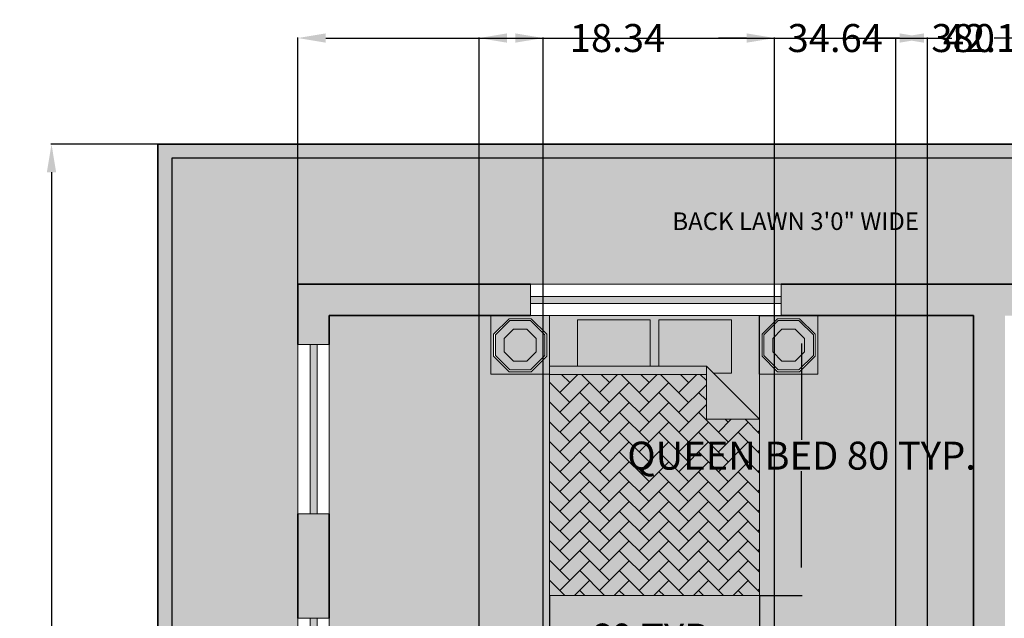
# Model space of a CAD drawing. Units: inches. Extents: x 389 to 971, y 148 to 870.
# Tile 11 of 14: x 389 to 670, y 699 to 870. Entities that reach past the tile are written whole.
import ezdxf

# ---------------------------------------------------------------- set-up
doc = ezdxf.new("R2010")
doc.units = ezdxf.units.IN
doc.header["$MEASUREMENT"] = 0
for name, color, linetype, lineweight in [('A-ANNO-DIMS', 2, 'Continuous', 18), ('A-ANNO-TEXT', 7, 'Continuous', 18), ('A-FLOR-BASE-PATT', 8, 'Continuous', 13), ('A-FURN', 8, 'Continuous', 18), ('A-FURN-PATT', 8, 'Continuous', 13), ('A-GLAZ', 4, 'Continuous', 18), ('A-WALL', 7, 'Continuous', 35), ('C-PROP', 7, 'Continuous', 35), ('L-GRND-BASE-PATT', 8, 'Continuous', 13), ('L-WALL', 7, 'Continuous', 30)]:
    doc.layers.add(name, color=color, linetype=linetype, lineweight=lineweight)
for name, color, linetype, lineweight, true_color in [('A-FURN-SURF-PATT', 9, 'Continuous', 13, 0xd6bdce), ('A-GLAZ-PATT', 251, 'Continuous', 13, 0x6d5f6c), ('A-WALL-PATT', 18, 'Continuous', 13, 0x000000), ('L-GRND-PATT', 39, 'Continuous', 13, 0x603913)]:
    doc.layers.add(name, color=color, linetype=linetype, lineweight=lineweight, true_color=true_color)
doc.styles.get("Standard").update_dxf_attribs({"font": 'arial.ttf'})
doc.dimstyles.get("Standard").update_dxf_attribs({"dimtxt": 8, "dimasz": 8, "dimexe": 0.18, "dimexo": 0.0625, "dimgap": 0.09, "dimtad": 0, "dimtih": 1, "dimtoh": 1, "dimdec": 0, "dimzin": 0, "dimdsep": 46, "dimlunit": 3, "dimtxsty": 'Standard', "dimcen": 0.09, "dimadec": 0, "dimazin": 0, "dimtfac": 1, "dimtdec": 0, "dimtofl": 0, "dimtmove": 0, "dimatfit": 3, "dimfxl": 1, "dimtolj": 1, "dimtzin": 0, "dimarcsym": 0})

# ---------------------------------------------------------------- blocks, each defined once
blk = doc.blocks.new('Bed - Queen')
for p, q in [((0, -80.00003), (0, 0)), ((0, 0), (59.99999, 0)), ((59.99999, 0), (59.99999, -80.00003)), ((7.99999, -1.2), (28.79998, -1.2)), ((7.99999, -14.4), (7.99999, -1.2)), ((28.79998, -1.2), (28.79998, -14.4)), ((31.19999, -1.2), (51.99999, -1.2)), ((31.19999, -14.4), (31.19999, -1.2)), ((51.99999, -1.2), (51.99999, -16.4)), ((0, -14.4), (44.8, -14.4)), ((44.8, -16.8), (0, -16.8)), ((59.99999, -29.6), (44.8, -14.4)), ((44.8, -14.4), (44.8, -29.6)), ((51.99999, -16.4), (46.79936, -16.4)), ((44.8, -29.6), (59.99999, -29.6)), ((59.99999, -80.00003), (0, -80.00003))]:
    blk.add_line(p, q)
blk = doc.blocks.new('Hot Tub')
for p, q in [((0, 0), (0, 69.12)), ((0, 69.12), (69.12, 69.12)), ((21.601, 65.456), (3.272, 47.128)), ((22.464, 63.396), (5.358, 46.29)), ((47.521, 65.456), (21.601, 65.456)), ((46.656, 63.396), (22.464, 63.396)), ((63.763, 46.29), (46.656, 63.396)), ((65.849, 47.128), (47.521, 65.456)), ((69.12, 69.12), (69.12, 0)), ((3.272, 47.128), (3.272, 21.208)), ((26.785, 53.097), (15.788, 42.101)), ((42.337, 53.097), (26.785, 53.097)), ((53.333, 42.101), (42.337, 53.097)), ((65.849, 21.208), (65.849, 47.128)), ((5.358, 46.29), (5.358, 22.098)), ((15.788, 42.101), (15.788, 26.549)), ((53.333, 26.549), (53.333, 42.101)), ((63.763, 22.098), (63.763, 46.29)), ((15.788, 26.549), (26.785, 15.552)), ((42.337, 15.552), (53.333, 26.549)), ((3.272, 21.208), (21.601, 2.88)), ((5.358, 22.098), (22.464, 4.992)), ((26.785, 15.552), (42.337, 15.552)), ((46.656, 4.992), (63.763, 22.098)), ((47.521, 2.88), (65.849, 21.208)), ((69.12, 0), (0, 0)), ((21.601, 2.88), (47.521, 2.88)), ((22.464, 4.992), (46.656, 4.992))]:
    blk.add_line(p, q)
blk = doc.blocks.new('*D24')
at = {"layer": 'A-ANNO-DIMS', "color": 0, "lineweight": -2, "transparency": 16777216}
for p, q in [((600.15, 785.64), (612.27, 785.64)), ((612.09, 777.64), (612.09, 750.12)), ((612.09, 713.64), (612.09, 741.17)), ((600.15, 705.64), (612.27, 705.64))]:
    blk.add_line(p, q, dxfattribs=at)
at = {"layer": 'A-ANNO-DIMS', "color": 0, "transparency": 16777216}
for points in [[(610.76, 777.64), (613.42, 777.64), (612.09, 785.64)], [(610.76, 713.64), (613.42, 713.64), (612.09, 705.64)]]:
    blk.add_solid(points, dxfattribs=at)
at = {"layer": 'Defpoints', "color": 0, "transparency": 16777216}
for p in [(600.09, 785.64), (612.09, 785.64), (600.09, 705.64)]:
    blk.add_point(p, dxfattribs=at)
at = {"layer": 'A-ANNO-DIMS', "color": 0, "transparency": 16777216, "insert": (612.09, 745.64), "char_height": 8, "attachment_point": 5}
blk.add_mtext('\\A1;QUEEN BED 80 TYP.', dxfattribs=at)
blk = doc.blocks.new('*D25')
at = {"layer": 'A-ANNO-DIMS', "color": 0, "lineweight": -2, "transparency": 16777216}
for p, q in [((540.09, 705.58), (540.09, 693.46)), ((600.09, 705.58), (600.09, 693.46)), ((548.09, 693.64), (550.51, 693.64)), ((592.09, 693.64), (589.67, 693.64))]:
    blk.add_line(p, q, dxfattribs=at)
at = {"layer": 'A-ANNO-DIMS', "color": 0, "transparency": 16777216}
for points in [[(548.09, 694.98), (548.09, 692.31), (540.09, 693.64)], [(592.09, 694.98), (592.09, 692.31), (600.09, 693.64)]]:
    blk.add_solid(points, dxfattribs=at)
at = {"layer": 'Defpoints', "color": 0, "transparency": 16777216}
for p in [(540.09, 705.64), (600.09, 705.64), (600.09, 693.64)]:
    blk.add_point(p, dxfattribs=at)
at = {"layer": 'A-ANNO-DIMS', "color": 0, "transparency": 16777216, "insert": (570.09, 693.64), "char_height": 8, "attachment_point": 5}
blk.add_mtext('\\A1;60 TYP.', dxfattribs=at)
blk = doc.blocks.new('*D45')
at = {"layer": 'A-ANNO-DIMS', "color": 0, "lineweight": -2, "transparency": 16777216}
for p, q in [((428.15, 834.64), (397.71, 834.64)), ((397.89, 826.64), (397.89, 538.82)), ((397.89, 242.64), (397.89, 530.47)), ((428.15, 234.64), (397.71, 234.64))]:
    blk.add_line(p, q, dxfattribs=at)
at = {"layer": 'A-ANNO-DIMS', "color": 0, "transparency": 16777216}
for points in [[(396.56, 826.64), (399.22, 826.64), (397.89, 834.64)], [(396.56, 242.64), (399.22, 242.64), (397.89, 234.64)]]:
    blk.add_solid(points, dxfattribs=at)
at = {"layer": 'Defpoints', "color": 0, "transparency": 16777216}
for p in [(397.89, 834.64), (428.22, 834.64), (428.22, 234.64)]:
    blk.add_point(p, dxfattribs=at)
at = {"layer": 'A-ANNO-DIMS', "color": 0, "transparency": 16777216, "insert": (397.89, 534.64), "char_height": 8, "attachment_point": 5}
blk.add_mtext('\\A1;600', dxfattribs=at)
blk = doc.blocks.new('*D46')
at = {"layer": 'A-ANNO-DIMS', "color": 0, "lineweight": -2, "transparency": 16777216}
for p, q in [((468.22, 794.71), (468.22, 865.15)), ((476.22, 864.97), (649.3, 864.97)), ((840.22, 864.97), (667.13, 864.97)), ((848.22, 834.71), (848.22, 865.15))]:
    blk.add_line(p, q, dxfattribs=at)
at = {"layer": 'A-ANNO-DIMS', "color": 0, "transparency": 16777216}
for points in [[(476.22, 866.3), (476.22, 863.64), (468.22, 864.97)], [(840.22, 866.3), (840.22, 863.64), (848.22, 864.97)]]:
    blk.add_solid(points, dxfattribs=at)
at = {"layer": 'Defpoints', "color": 0, "transparency": 16777216}
for p in [(848.22, 864.97), (848.22, 834.64), (468.22, 794.64)]:
    blk.add_point(p, dxfattribs=at)
at = {"layer": 'A-ANNO-DIMS', "color": 0, "transparency": 16777216, "insert": (658.22, 864.97), "char_height": 8, "attachment_point": 5}
blk.add_mtext('\\A1;380', dxfattribs=at)
blk = doc.blocks.new('*D49')
at = {"layer": 'A-ANNO-DIMS', "color": 0, "lineweight": -2, "transparency": 16777216}
for p, q in [((519.98, 632.71), (519.98, 865.15)), ((527.98, 864.97), (530.32, 864.97)), ((538.32, 632.71), (538.32, 865.15)), ((538.32, 864.97), (546.32, 864.97))]:
    blk.add_line(p, q, dxfattribs=at)
at = {"layer": 'A-ANNO-DIMS', "color": 0, "transparency": 16777216}
for points in [[(527.98, 866.3), (527.98, 863.64), (519.98, 864.97)], [(530.32, 866.3), (530.32, 863.64), (538.32, 864.97)]]:
    blk.add_solid(points, dxfattribs=at)
at = {"layer": 'Defpoints', "color": 0, "transparency": 16777216}
for p in [(538.32, 864.97), (519.98, 632.64), (538.32, 632.64)]:
    blk.add_point(p, dxfattribs=at)
at = {"layer": 'A-ANNO-DIMS', "color": 0, "transparency": 16777216, "insert": (559.52, 864.97), "char_height": 8, "attachment_point": 5}
blk.add_mtext('\\A1;18.34', dxfattribs=at)
blk = doc.blocks.new('*D51')
at = {"layer": 'A-ANNO-DIMS', "color": 0, "lineweight": -2, "transparency": 16777216}
for p, q in [((596.39, 864.97), (588.39, 864.97)), ((604.39, 354.78), (604.39, 865.15)), ((639.03, 354.78), (639.03, 865.15)), ((647.03, 864.97), (655.03, 864.97))]:
    blk.add_line(p, q, dxfattribs=at)
at = {"layer": 'A-ANNO-DIMS', "color": 0, "transparency": 16777216}
for points in [[(596.39, 866.3), (596.39, 863.64), (604.39, 864.97)], [(647.03, 866.3), (647.03, 863.64), (639.03, 864.97)]]:
    blk.add_solid(points, dxfattribs=at)
at = {"layer": 'Defpoints', "color": 0, "transparency": 16777216}
for p in [(639.03, 864.97), (604.39, 354.72), (639.03, 354.72)]:
    blk.add_point(p, dxfattribs=at)
at = {"layer": 'A-ANNO-DIMS', "color": 0, "transparency": 16777216, "insert": (621.71, 864.97), "char_height": 8, "attachment_point": 5}
blk.add_mtext('\\A1;34.64', dxfattribs=at)
blk = doc.blocks.new('*D52')
at = {"layer": 'A-ANNO-DIMS', "color": 0, "lineweight": -2, "transparency": 16777216}
for p, q in [((640.06, 864.97), (632.06, 864.97)), ((648.06, 388.98), (648.06, 865.15)), ((690.22, 388.98), (690.22, 865.15)), ((698.22, 864.97), (706.22, 864.97))]:
    blk.add_line(p, q, dxfattribs=at)
at = {"layer": 'A-ANNO-DIMS', "color": 0, "transparency": 16777216}
for points in [[(640.06, 866.3), (640.06, 863.64), (648.06, 864.97)], [(698.22, 866.3), (698.22, 863.64), (690.22, 864.97)]]:
    blk.add_solid(points, dxfattribs=at)
at = {"layer": 'Defpoints', "color": 0, "transparency": 16777216}
for p in [(690.22, 864.97), (648.06, 388.92), (690.22, 388.92)]:
    blk.add_point(p, dxfattribs=at)
at = {"layer": 'A-ANNO-DIMS', "color": 0, "transparency": 16777216, "insert": (669.14, 864.97), "char_height": 8, "attachment_point": 5}
blk.add_mtext('\\A1;42.155', dxfattribs=at)

msp = doc.modelspace()

# ---------------------------------------------------------------- hatches: boundary and pattern name
at = {"layer": 'A-FLOR-BASE-PATT'}
h = msp.add_hatch(color=256, dxfattribs=at)
h.dxf.hatch_style = 1
h.paths.add_polyline_path([(651.6417, 675.6801), (651.6417, 675.7122), (653.109, 675.7122), (653.109, 641.6445), (661.216, 641.6445), (661.216, 785.6445), (616.7487, 785.6445), (616.7487, 768.9039), (600.0901, 768.9039), (600.0901, 705.6445), (540.0901, 705.6445), (540.0901, 768.9039), (523.3494, 768.9039), (523.3494, 785.6445), (477.216, 785.6445), (477.216, 777.4428), (477.216, 728.9805), (477.216, 699.1491), (477.216, 651.2738), (477.216, 641.6445), (519.983, 641.6445), (519.983, 632.5593), (521.3203, 632.5593), (521.3203, 614.2674, 0.39433689), (538.3235, 632.6445), (538.3237, 632.6445), (538.3237, 637.1445), (538.3237, 641.6445), (619.5719, 641.6445), (619.5719, 642.1751, -0.40145271)])
h.paths.add_polyline_path([(546.1308, 677.2872), (587.0907, 677.2872), (587.0907, 696.0138), (546.1308, 696.0138)], flags=24)
at = {"layer": 'A-FURN-PATT'}
h = msp.add_hatch(dxfattribs=at)
h.set_pattern_fill('AR-HBONE', color=256)
h.paths.add_polyline_path([(540.0901, 705.6445), (600.0901, 705.6445), (600.0901, 756.0445), (584.8901, 756.0445), (584.8901, 768.8445), (540.0901, 768.8445)])
at = {"layer": 'A-FURN-SURF-PATT'}
h = msp.add_hatch(color=256, dxfattribs=at)
h.dxf.hatch_style = 1
h.paths.add_polyline_path([(540.0901, 785.6445), (533.9078, 785.6445), (523.3494, 785.6445), (523.3494, 768.9039), (540.0901, 768.9039)])
h.paths.add_polyline_path([(528.5811, 784.7571), (534.8589, 784.7571), (539.2979, 780.3181), (539.2979, 774.0404), (534.8589, 769.6014), (528.5811, 769.6014), (524.1419, 774.0404), (524.1419, 780.3181)], flags=16)
h.paths.add_polyline_path([(528.7902, 784.2582), (534.6494, 784.2582), (538.7927, 780.1152), (538.7927, 774.2559), (534.6494, 770.1129), (528.7902, 770.1129), (524.6471, 774.2559), (524.6471, 780.1152)], flags=0)
h.paths.add_polyline_path([(529.8367, 781.7638), (533.6033, 781.7638), (536.2665, 779.1006), (536.2665, 775.3339), (533.6033, 772.6705), (529.8367, 772.6705), (527.1732, 775.3339), (527.1732, 779.1006)], flags=0)
h = msp.add_hatch(color=256, dxfattribs=at)
h.dxf.hatch_style = 1
h.paths.add_polyline_path([(548.0901, 784.4445), (568.8901, 784.4445), (568.8901, 771.2445), (571.2901, 771.2445), (571.2901, 784.4445), (592.0901, 784.4445), (592.0901, 769.2445), (586.8901, 769.2445), (600.0901, 756.0445), (600.0901, 768.9039), (600.008, 768.9039), (600.008, 785.6445), (540.0901, 785.6445), (540.0901, 771.2445), (548.0901, 771.2445)])
h = msp.add_hatch(color=256, dxfattribs=at)
h.dxf.hatch_style = 1
h.paths.add_polyline_path([(616.7487, 785.6445), (606.2724, 785.6445), (600.0901, 785.6445), (600.0901, 768.9039), (616.7487, 768.9039)])
h.paths.add_polyline_path([(605.2397, 784.7571), (611.5174, 784.7571), (615.9564, 780.3181), (615.9564, 774.0404), (611.5174, 769.6014), (605.2397, 769.6014), (600.8005, 774.0404), (600.8005, 780.3181)], flags=16)
h.paths.add_polyline_path([(605.4487, 784.2582), (611.3079, 784.2582), (615.4512, 780.1152), (615.4512, 774.2559), (611.3079, 770.1129), (605.4487, 770.1129), (601.3057, 774.2559), (601.3057, 780.1152)], flags=0)
h.paths.add_polyline_path([(606.4952, 781.7638), (610.2619, 781.7638), (612.9251, 779.1006), (612.9251, 775.3339), (610.2619, 772.6705), (606.4952, 772.6705), (603.8318, 775.3339), (603.8318, 779.1006)], flags=0)
h = msp.add_hatch(color=256, dxfattribs=at)
h.dxf.hatch_style = 1
h.paths.add_polyline_path([(529.8367, 772.6705), (533.6033, 772.6705), (536.2665, 775.3339), (536.2665, 779.1006), (533.6033, 781.7638), (529.8367, 781.7638), (527.1732, 779.1006), (527.1732, 775.3339)], flags=16)
h.paths.add_polyline_path([(534.6494, 770.1129), (538.7927, 774.2559), (538.7927, 780.1152), (534.6494, 784.2582), (528.7902, 784.2582), (524.6471, 780.1152), (524.6471, 774.2559), (528.7902, 770.1129)])
h = msp.add_hatch(color=256, dxfattribs=at)
h.dxf.hatch_style = 1
h.paths.add_polyline_path([(529.8367, 772.6705), (533.6033, 772.6705), (536.2665, 775.3339), (536.2665, 779.1006), (533.6033, 781.7638), (529.8367, 781.7638), (527.1732, 779.1006), (527.1732, 775.3339)])
h = msp.add_hatch(color=256, dxfattribs=at)
h.dxf.hatch_style = 1
h.paths.add_polyline_path([(568.8901, 771.2445), (568.8901, 784.4445), (548.0901, 784.4445), (548.0901, 771.2445)])
h = msp.add_hatch(color=256, dxfattribs=at)
h.dxf.hatch_style = 1
h.paths.add_polyline_path([(584.8901, 771.2445), (586.8901, 769.2445), (592.0901, 769.2445), (592.0901, 784.4445), (571.2901, 784.4445), (571.2901, 771.2445)])
h = msp.add_hatch(color=256, dxfattribs=at)
h.dxf.hatch_style = 1
h.paths.add_polyline_path([(610.2619, 772.6705), (612.9251, 775.3339), (612.9251, 779.1006), (610.2619, 781.7638), (606.4952, 781.7638), (603.8318, 779.1006), (603.8318, 775.3339), (606.4952, 772.6705)], flags=16)
h.paths.add_polyline_path([(611.3079, 770.1129), (615.4512, 774.2559), (615.4512, 780.1152), (611.3079, 784.2582), (605.4487, 784.2582), (601.3057, 780.1152), (601.3057, 774.2559), (605.4487, 770.1129)])
h = msp.add_hatch(color=256, dxfattribs=at)
h.dxf.hatch_style = 1
h.paths.add_polyline_path([(612.9251, 775.3339), (612.9251, 779.1006), (610.2619, 781.7638), (606.4952, 781.7638), (603.8318, 779.1006), (603.8318, 775.3339), (606.4952, 772.6705), (610.2619, 772.6705)])
h = msp.add_hatch(color=256, dxfattribs=at)
h.dxf.hatch_style = 1
h.paths.add_polyline_path([(540.0901, 771.2445), (540.0901, 768.8445), (584.8901, 768.8445), (584.8901, 771.2445)])
h = msp.add_hatch(color=256, dxfattribs=at)
h.dxf.hatch_style = 1
h.paths.add_polyline_path([(584.8901, 756.0445), (600.0901, 756.0445), (584.8901, 771.2445)])
h = msp.add_hatch(color=256, dxfattribs=at)
h.dxf.hatch_style = 1
h.paths.add_polyline_path([(540.0901, 705.6445), (600.0901, 705.6445), (600.0901, 756.0445), (584.8901, 756.0445), (584.8901, 768.8445), (540.0901, 768.8445)])
at = {"layer": 'A-GLAZ-PATT'}
h = msp.add_hatch(color=256, dxfattribs=at)
h.dxf.hatch_style = 1
h.paths.add_polyline_path([(534.7176, 791.1445), (534.7176, 789.1445), (606.2724, 789.1445), (606.2724, 791.1445)])
h = msp.add_hatch(color=256, dxfattribs=at)
h.dxf.hatch_style = 1
h.paths.add_polyline_path([(473.716, 777.4428), (471.716, 777.4428), (471.716, 728.9805), (473.716, 728.9805)])
h = msp.add_hatch(color=256, dxfattribs=at)
h.dxf.hatch_style = 1
h.paths.add_polyline_path([(473.716, 699.1491), (471.716, 699.1491), (471.716, 651.2738), (473.716, 651.2738)])
at = {"layer": 'A-WALL-PATT'}
h = msp.add_hatch(color=256, dxfattribs=at)
h.dxf.hatch_style = 1
h.paths.add_polyline_path([(432.216, 434.6445), (436.3673, 434.6445), (436.3673, 443.6445), (432.216, 443.6445), (432.216, 830.6445), (746.216, 830.6445), (746.216, 823.8175), (755.216, 823.8175), (755.216, 825.6445), (839.216, 825.6445), (839.216, 803.5176), (839.216, 741.6445), (755.216, 741.6445), (755.216, 748.4596), (755.1859, 748.4596), (750.716, 748.4596), (746.216, 748.4596), (746.216, 732.6445), (839.216, 732.6445), (839.216, 600.6445), (708.5171, 600.6445), (708.5171, 596.1445), (708.5171, 591.6445), (794.216, 591.6445), (794.216, 587.4291), (803.216, 587.4291), (803.216, 591.6445), (839.216, 591.6445), (839.216, 466.6012), (803.216, 466.6012), (803.216, 471.0309), (794.216, 471.0309), (794.216, 466.6012), (784.6145, 466.6012), (784.6145, 457.6012), (839.216, 457.6012), (839.216, 447.6445), (839.216, 294.6445), (810.0514, 294.6445), (810.0514, 285.6445), (839.216, 285.6445), (839.216, 238.6445), (590.216, 238.6445), (590.216, 234.6445), (848.216, 234.6445), (848.216, 834.6445), (428.216, 834.6445), (428.216, 234.6445), (437.216, 234.6445), (437.216, 243.6445), (432.216, 243.6445)])
h = msp.add_hatch(color=256, dxfattribs=at)
h.dxf.hatch_style = 1
h.paths.add_polyline_path([(468.216, 777.4428), (477.216, 777.4428), (477.216, 785.6445), (534.7176, 785.6445), (534.7176, 794.6445), (533.9078, 794.6445), (468.216, 794.6445)])
h = msp.add_hatch(color=256, dxfattribs=at)
h.dxf.hatch_style = 1
h.paths.add_polyline_path([(661.216, 785.6445), (661.216, 641.6445), (653.109, 641.6445), (653.109, 637.1445), (653.109, 632.6445), (661.216, 632.6445), (661.216, 591.6445), (676.6391, 591.6445), (676.6391, 600.6445), (670.216, 600.6445), (670.216, 785.6445), (685.2392, 785.6445), (685.2392, 794.6445), (662.4125, 794.6445), (606.2724, 794.6445), (606.2724, 785.6445), (616.7487, 785.6445)])
h = msp.add_hatch(color=256, dxfattribs=at)
h.dxf.hatch_style = 1
h.paths.add_polyline_path([(468.216, 699.1491), (477.216, 699.1491), (477.216, 728.9805), (468.216, 728.9805)])
at = {"layer": 'L-GRND-BASE-PATT'}
h = msp.add_hatch(color=256, dxfattribs=at)
h.dxf.hatch_style = 1
h.paths.add_polyline_path([(468.216, 560.6445), (502.387, 560.6445), (502.387, 585.4344), (502.387, 613.354), (502.387, 632.6445), (468.216, 632.6445), (468.216, 651.2738), (468.216, 699.1491), (468.216, 728.9805), (468.216, 777.4428), (468.216, 794.6445), (534.7176, 794.6445), (606.2724, 794.6445), (685.2392, 794.6445), (734.7772, 794.6445), (746.216, 794.6445), (746.216, 796.191), (746.216, 823.8175), (746.216, 830.6445), (432.216, 830.6445), (432.216, 443.6445), (468.216, 443.6445), (468.216, 452.1978), (468.216, 490.1255), (468.216, 508.3496), (468.216, 543.0462)])
h.paths.add_polyline_path([(456.8918, 600.1849), (456.8918, 677.4216), (446.55, 677.4216), (446.55, 600.1849)], flags=24)
h.paths.add_polyline_path([(573.4326, 807.2886), (651.063, 807.2886), (651.063, 817.6304), (573.4326, 817.6304)], flags=24)
at = {"layer": 'L-GRND-PATT'}
h = msp.add_hatch(dxfattribs=at)
h.set_pattern_fill('EARTH', color=256, angle=45)
h.set_pattern_definition([(45, (0, 0), (0, 8.980256), [6.35, -6.35]), (45, (-1.684, 1.684), (0, 8.980256), [6.35, -6.35]), (45, (-3.3676, 3.3676), (0, 8.980256), [6.35, -6.35]), (135, (-3.3676, 4.49), (-8.980256, 0), [6.35, -6.35]), (135, (-1.684, 6.174), (-8.980256, 0), [6.35, -6.35]), (135, (0, 7.858), (-8.980256, 0), [6.35, -6.35])])
h.paths.add_polyline_path([(468.216, 560.6445), (502.387, 560.6445), (502.387, 585.4344), (502.387, 613.354), (502.387, 632.6445), (468.216, 632.6445), (468.216, 651.2738), (468.216, 699.1491), (468.216, 728.9805), (468.216, 777.4428), (468.216, 794.6445), (534.7176, 794.6445), (606.2724, 794.6445), (685.2392, 794.6445), (734.7772, 794.6445), (746.216, 794.6445), (746.216, 796.191), (746.216, 823.8175), (746.216, 830.6445), (432.216, 830.6445), (432.216, 443.6445), (468.216, 443.6445), (468.216, 452.1978), (468.216, 490.1255), (468.216, 508.3496), (468.216, 543.0462)])
h.paths.add_polyline_path([(456.8918, 600.1849), (456.8918, 677.4216), (446.55, 677.4216), (446.55, 600.1849)], flags=24)
h.paths.add_polyline_path([(573.4326, 807.2886), (651.063, 807.2886), (651.063, 817.6304), (573.4326, 817.6304)], flags=24)

# ---------------------------------------------------------------- linework, layer by layer
at = {"layer": 'A-GLAZ'}
for p, q in [((533.9078, 794.6445), (606.2724, 794.6445)), ((534.7176, 785.6445), (534.7176, 794.6445)), ((606.2724, 785.6445), (606.2724, 794.6445)), ((606.2724, 794.6445), (606.2724, 785.6445)), ((662.4125, 794.6445), (734.7772, 794.6445)), ((534.7176, 791.1445), (606.2724, 791.1445)), ((534.7176, 789.1445), (606.2724, 789.1445)), ((533.9078, 785.6445), (606.2724, 785.6445)), ((477.216, 777.4428), (468.216, 777.4428)), ((468.216, 777.4428), (468.216, 728.9805)), ((471.716, 777.4428), (471.716, 728.9805)), ((473.716, 777.4428), (473.716, 728.9805)), ((477.216, 777.4428), (477.216, 728.9805)), ((477.216, 728.9805), (468.216, 728.9805)), ((477.216, 699.1491), (468.216, 699.1491)), ((468.216, 699.1491), (468.216, 651.2738)), ((471.716, 699.1491), (471.716, 651.2738)), ((473.716, 699.1491), (473.716, 651.2738)), ((477.216, 699.1491), (477.216, 651.2738))]:
    msp.add_line(p, q, dxfattribs=at)
at = {"layer": 'A-WALL'}
for p, q in [((468.216, 794.6445), (468.216, 777.4428)), ((534.7176, 794.6445), (468.216, 794.6445)), ((685.2392, 794.6445), (606.2724, 794.6445)), ((477.216, 785.6445), (477.216, 777.4428)), ((534.7176, 785.6445), (477.216, 785.6445)), ((661.216, 785.6445), (606.2724, 785.6445)), ((661.216, 785.6445), (661.216, 641.6445)), ((468.216, 728.9805), (468.216, 699.1491)), ((477.216, 728.9805), (477.216, 699.1491))]:
    msp.add_line(p, q, dxfattribs=at)
at = {"layer": 'C-PROP'}
for p, q in [((848.216, 834.6445), (428.216, 834.6445)), ((428.216, 834.6445), (428.216, 234.6445))]:
    msp.add_line(p, q, dxfattribs=at)
at = {"layer": 'L-WALL'}
for p, q in [((432.216, 830.6445), (432.216, 443.6445)), ((746.216, 830.6445), (432.216, 830.6445))]:
    msp.add_line(p, q, dxfattribs=at)

# ---------------------------------------------------------------- block references
at = {"layer": 'A-FURN', "xscale": 0.2421970890605389, "yscale": 0.2421970890605389, "zscale": 0.2421970890605389}
for p in [(523.3494, 768.9039), (600.008, 768.9039)]:
    msp.add_blockref('Hot Tub', p, dxfattribs=at)
at = {"layer": 'A-FURN'}
msp.add_blockref('Bed - Queen', (540.0901, 785.6445), dxfattribs=at)

# ---------------------------------------------------------------- texts
at = {"layer": 'A-ANNO-TEXT', "insert": (575.2008, 815.1331), "char_height": 5.018573, "attachment_point": 1}
msp.add_mtext_dynamic_manual_height_columns('BACK LAWN 3\'0" WIDE', width=113.900213, gutter_width=25.0929, heights=[0], dxfattribs=at)

# ---------------------------------------------------------------- dimensions: what is measured, and where the dimension line sits
at = {"layer": 'A-ANNO-DIMS'}
for base, p1, p2, override, picture, middle in [((848.216, 864.9695), (468.216, 794.6445), (848.216, 834.6445), {"dimdec": 0, "dimlfac": 1, "dimrnd": 0, "dimzin": 0, "dimdsep": 46, "dimlunit": 2}, '*D46', (658.216, 864.9695)), ((538.3237, 864.9695), (519.983, 632.6445), (538.3237, 632.6445), {"dimdec": 2, "dimlfac": 1, "dimrnd": 0, "dimzin": 0, "dimdsep": 46, "dimlunit": 2}, '*D49', (559.5188, 864.9695)), ((639.0296, 864.9695), (604.387, 354.7191), (639.0296, 354.7191), {"dimdec": 2, "dimlfac": 1, "dimrnd": 0, "dimzin": 0, "dimdsep": 46, "dimlunit": 2}, '*D51', (621.7083, 864.9695)), ((690.216, 864.9695), (648.061, 388.9189), (690.216, 388.9189), {"dimdec": 3, "dimlfac": 1, "dimrnd": 0, "dimzin": 0, "dimdsep": 46, "dimlunit": 2}, '*D52', (669.1385, 864.9695))]:
    dim = msp.add_linear_dim(base=base, p1=p1, p2=p2, dimstyle='Standard', override=override, dxfattribs=at)
    dim.commit()
    dim.dimension.update_dxf_attribs({"geometry": picture, "text_midpoint": middle})
dim = msp.add_linear_dim(base=(397.891, 834.6445), p1=(428.216, 234.6445), p2=(428.216, 834.6445), angle=90, dimstyle='Standard', override={"dimdec": 0, "dimlfac": 1, "dimrnd": 0, "dimzin": 0, "dimdsep": 46, "dimlunit": 2}, dxfattribs=at)
dim.commit()
dim.dimension.update_dxf_attribs({"geometry": '*D45', "text_midpoint": (397.891, 534.6445)})
dim = msp.add_linear_dim(base=(612.0901, 785.6445), p1=(600.0901, 705.6445), p2=(600.0901, 785.6445), angle=90, text='QUEEN BED <> TYP.', dimstyle='Standard', override={"dimdec": 0, "dimlfac": 1, "dimrnd": 0, "dimzin": 0, "dimdsep": 46, "dimlunit": 2}, dxfattribs=at)
dim.commit()
dim.dimension.update_dxf_attribs({"geometry": '*D24', "text_midpoint": (612.0901, 745.6445)})
dim = msp.add_linear_dim(base=(600.0901, 693.6445), p1=(540.0901, 705.6445), p2=(600.0901, 705.6445), text='<> TYP.', dimstyle='Standard', override={"dimdec": 0, "dimlfac": 1, "dimrnd": 0, "dimzin": 0, "dimdsep": 46, "dimlunit": 2}, dxfattribs=at)
dim.commit()
dim.dimension.update_dxf_attribs({"geometry": '*D25', "text_midpoint": (570.0901, 693.6445)})

doc.saveas('drawing.dxf')
